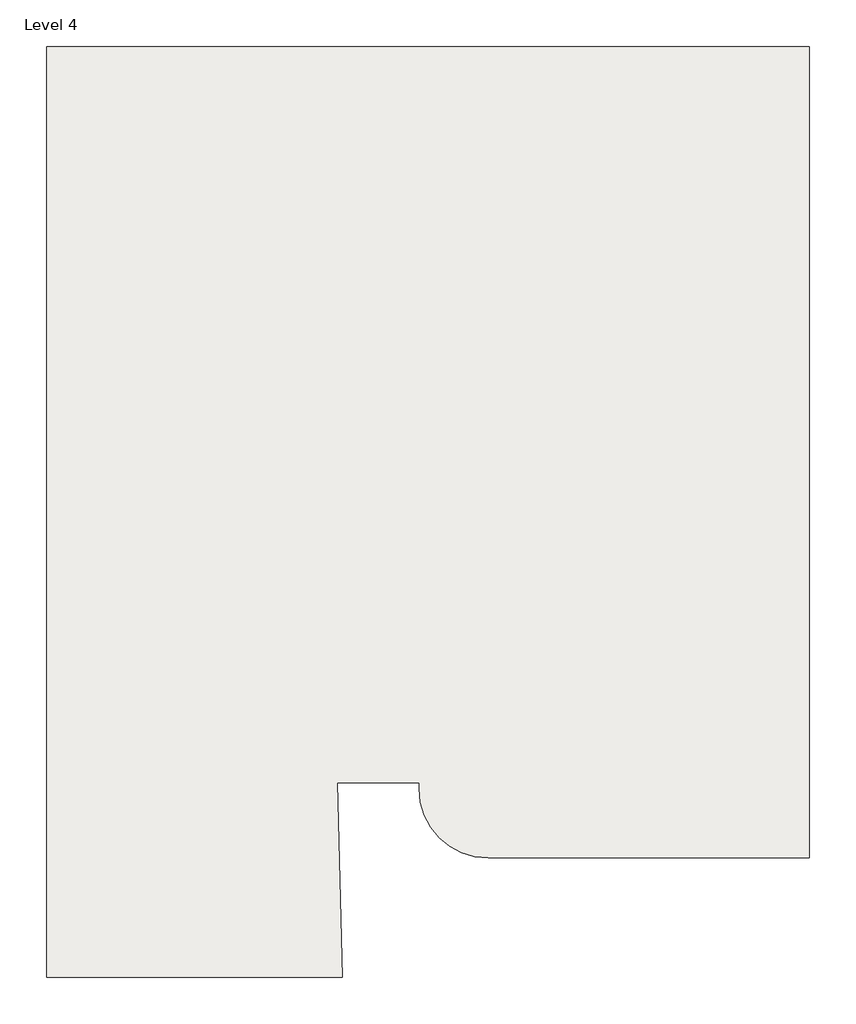
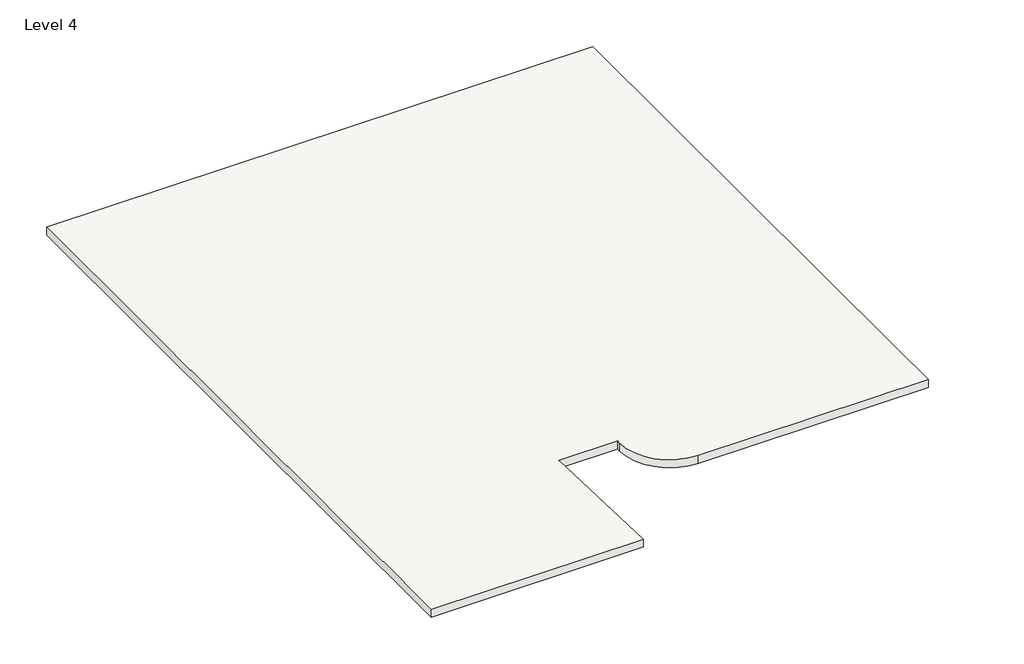
# One storey: 1 slab.
"""IFC4 building model written with IfcOpenShell, lengths in millimetres."""

from ifc_helpers import new_model, si_unit, point, frame, frame_2d, origin, place, context, project, spatial, polyline, circle_curve, trimmed, segment, composite_curve, outline, extrude, element, save

model = new_model("IFC4")

# Units and contexts
model_context = context("Model", 3, world=origin())
ifc_project = project(units=[si_unit("LENGTHUNIT", "METRE", prefix="MILLI")], contexts=[model_context])

# Site, building, storey
site = spatial("IfcSite", under=ifc_project)
building = spatial("IfcBuilding", under=site)
storey = spatial("IfcBuildingStorey", under=building, Name="Level 4", Elevation=10058.4)

# Slab
placement = place(None, origin())
element("IfcSlab", 1, ObjectType="Generic - 12\"", at=placement, inside=storey, context=model_context, shape_type="SweptSolid", body=[
    extrude(outline(composite_curve([segment(polyline([(-10290.7310626, -15454.510779), (-10290.7310626, 9081.889221), (9814.2068176, 9081.889221), (9814.2068176, -10323.710779), (9814.2068176, -12304.910779), (1356.0068176, -12304.910779)]), True, "CONTINUOUS"), segment(trimmed(circle_curve(frame_2d((1356.0068176, -10476.110779)), 1828.8), [point((1356.0068176, -12304.910779))], [point((-472.7931824, -10476.110779))], False, "CARTESIAN"), True, "CONTINUOUS"), segment(polyline([(-472.7931824, -10476.110779), (-472.7931824, -10323.710779), (-2631.7931824, -10323.710779), (-2493.6095113, -15454.510779), (-10290.7310626, -15454.510779)]), True, "CONTINUOUS")], self_intersect=False)), frame((0.0, 0.0, 9753.6), z_axis=(0.0, 0.0, 1.0), x_axis=(1.0, 0.0, 0.0)), (0.0, 0.0, 1.0), 304.8),
])

save(model, "model.ifc")

# Revit data of these elements
# Type "Generic - 12\""
#   Assembly Code = "B1010"
#   Function = 0
#   Layers, outside or top first: 1' - 0" no material (function 1)
# Element 1 (IfcSlab, "Generic - 12\"")
#   built-in parameter 1001955 = -1.5708 (stored number, unit not read)
#   Height Offset From Level = 0' - 0"
#   Phase Created = New Construction
#   Materials on its faces: "Default Floor", "Brick, Soldier Course"
# Materials
#   "Default Floor": colour RGB 128 128 128, transparency 0, Cost = 0
#   "Brick, Soldier Course": class "Masonry", colour RGB 170 98 104, transparency 0, Description = "Common brick soldier coursed", Cost = 0
